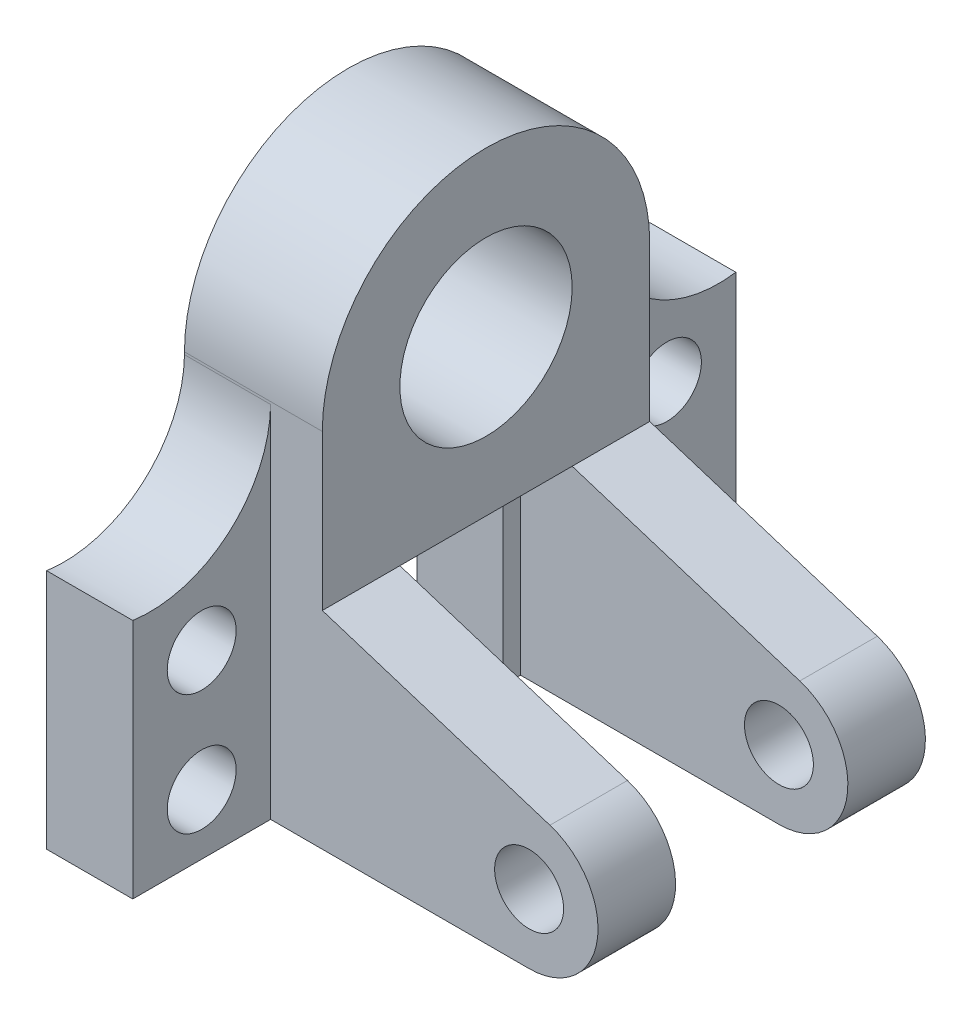
ISO-10303-21;
HEADER;
FILE_DESCRIPTION(('STEP AP214'),'2;1');
FILE_NAME('part.step','',(''),(''),'','','');
FILE_SCHEMA(('AUTOMOTIVE_DESIGN { 1 0 10303 214 1 1 1 1 }'));
ENDSEC;
DATA;
#1=APPLICATION_CONTEXT('core data for automotive mechanical design processes');
#2=APPLICATION_PROTOCOL_DEFINITION('international standard','automotive_design',2000,#1);
#3=PRODUCT_CONTEXT('',#1,'mechanical');
#4=PRODUCT('Part','Part','',(#3));
#5=PRODUCT_RELATED_PRODUCT_CATEGORY('part','',(#4));
#6=PRODUCT_DEFINITION_FORMATION('','',#4);
#7=PRODUCT_DEFINITION_CONTEXT('part definition',#1,'design');
#8=PRODUCT_DEFINITION('design','',#6,#7);
#9=PRODUCT_DEFINITION_SHAPE('','',#8);
#10=(LENGTH_UNIT() NAMED_UNIT(*) SI_UNIT(.MILLI.,.METRE.));
#11=(NAMED_UNIT(*) PLANE_ANGLE_UNIT() SI_UNIT($,.RADIAN.));
#12=(NAMED_UNIT(*) SI_UNIT($,.STERADIAN.) SOLID_ANGLE_UNIT());
#13=UNCERTAINTY_MEASURE_WITH_UNIT(LENGTH_MEASURE(1.E-05),#10,'distance_accuracy_value','');
#14=(GEOMETRIC_REPRESENTATION_CONTEXT(3) GLOBAL_UNCERTAINTY_ASSIGNED_CONTEXT((#13)) GLOBAL_UNIT_ASSIGNED_CONTEXT((#10,
#11,#12)) REPRESENTATION_CONTEXT('',''));
#15=CARTESIAN_POINT('',(0.,0.,0.));
#16=DIRECTION('',(0.,0.,1.));
#17=DIRECTION('',(1.,0.,0.));
#18=AXIS2_PLACEMENT_3D('',#15,#16,#17);
#19=CARTESIAN_POINT('',(16.,-36.,38.));
#20=DIRECTION('',(0.,1.,0.));
#21=DIRECTION('',(0.,0.,1.));
#22=AXIS2_PLACEMENT_3D('',#19,#20,#21);
#23=PLANE('',#22);
#24=DIRECTION('',(-1.,0.,0.));
#25=VECTOR('',#24,1.);
#26=CARTESIAN_POINT('',(4.,-36.,16.));
#27=LINE('',#26,#25);
#28=CARTESIAN_POINT('',(4.,-36.,16.));
#29=VERTEX_POINT('',#28);
#30=CARTESIAN_POINT('',(-16.,-36.,16.));
#31=VERTEX_POINT('',#30);
#32=EDGE_CURVE('E401',#29,#31,#27,.T.);
#33=ORIENTED_EDGE('',*,*,#32,.T.);
#34=DIRECTION('',(0.,0.,-1.));
#35=VECTOR('',#34,1.);
#36=CARTESIAN_POINT('',(-16.,-36.,38.));
#37=LINE('',#36,#35);
#38=CARTESIAN_POINT('',(-16.,-36.,-16.));
#39=VERTEX_POINT('',#38);
#40=EDGE_CURVE('E61',#31,#39,#37,.T.);
#41=ORIENTED_EDGE('',*,*,#40,.T.);
#42=DIRECTION('',(-1.,0.,0.));
#43=VECTOR('',#42,1.);
#44=CARTESIAN_POINT('',(4.,-36.,-16.));
#45=LINE('',#44,#43);
#46=CARTESIAN_POINT('',(4.,-36.,-16.));
#47=VERTEX_POINT('',#46);
#48=EDGE_CURVE('E57',#47,#39,#45,.T.);
#49=ORIENTED_EDGE('',*,*,#48,.F.);
#50=DIRECTION('',(0.,0.,1.));
#51=VECTOR('',#50,1.);
#52=CARTESIAN_POINT('',(4.,-36.,0.));
#53=LINE('',#52,#51);
#54=CARTESIAN_POINT('',(4.,-36.,-20.));
#55=VERTEX_POINT('',#54);
#56=EDGE_CURVE('E387',#55,#47,#53,.T.);
#57=ORIENTED_EDGE('',*,*,#56,.F.);
#58=DIRECTION('',(1.,0.,0.));
#59=VECTOR('',#58,1.);
#60=CARTESIAN_POINT('',(0.,-36.,-20.));
#61=LINE('',#60,#59);
#62=CARTESIAN_POINT('',(16.,-36.,-20.));
#63=VERTEX_POINT('',#62);
#64=EDGE_CURVE('E363',#55,#63,#61,.T.);
#65=ORIENTED_EDGE('',*,*,#64,.T.);
#66=DIRECTION('',(0.,0.,-1.));
#67=VECTOR('',#66,1.);
#68=CARTESIAN_POINT('',(16.,-36.,38.));
#69=LINE('',#68,#67);
#70=CARTESIAN_POINT('',(16.,-36.,20.));
#71=VERTEX_POINT('',#70);
#72=EDGE_CURVE('E250',#71,#63,#69,.T.);
#73=ORIENTED_EDGE('',*,*,#72,.F.);
#74=DIRECTION('',(1.,0.,0.));
#75=VECTOR('',#74,1.);
#76=CARTESIAN_POINT('',(0.,-36.,20.));
#77=LINE('',#76,#75);
#78=CARTESIAN_POINT('',(4.,-36.,20.));
#79=VERTEX_POINT('',#78);
#80=EDGE_CURVE('E208',#79,#71,#77,.T.);
#81=ORIENTED_EDGE('',*,*,#80,.F.);
#82=DIRECTION('',(0.,0.,-1.));
#83=VECTOR('',#82,1.);
#84=CARTESIAN_POINT('',(4.,-36.,0.));
#85=LINE('',#84,#83);
#86=EDGE_CURVE('E200',#79,#29,#85,.T.);
#87=ORIENTED_EDGE('',*,*,#86,.T.);
#88=EDGE_LOOP('',(#33,#41,#49,#57,#65,#73,#81,#87));
#89=FACE_BOUND('',#88,.T.);
#90=ADVANCED_FACE('F41',(#89),#23,.F.);
#91=CARTESIAN_POINT('',(0.,0.,20.));
#92=DIRECTION('',(0.,0.,1.));
#93=DIRECTION('',(1.,0.,0.));
#94=AXIS2_PLACEMENT_3D('',#91,#92,#93);
#95=PLANE('',#94);
#96=CARTESIAN_POINT('',(64.,-68.,20.));
#97=DIRECTION('',(0.,0.,1.));
#98=DIRECTION('',(1.,0.,0.));
#99=AXIS2_PLACEMENT_3D('',#96,#97,#98);
#100=CIRCLE('',#99,7.99999999999999);
#101=CARTESIAN_POINT('',(72.,-68.,20.));
#102=VERTEX_POINT('',#101);
#103=EDGE_CURVE('E210',#102,#102,#100,.T.);
#104=ORIENTED_EDGE('',*,*,#103,.T.);
#105=EDGE_LOOP('',(#104));
#106=FACE_BOUND('',#105,.T.);
#107=DIRECTION('',(0.,1.,0.));
#108=VECTOR('',#107,1.);
#109=CARTESIAN_POINT('',(4.,0.,20.));
#110=LINE('',#109,#108);
#111=CARTESIAN_POINT('',(4.,-84.,20.));
#112=VERTEX_POINT('',#111);
#113=EDGE_CURVE('E191',#112,#79,#110,.T.);
#114=ORIENTED_EDGE('',*,*,#113,.T.);
#115=ORIENTED_EDGE('',*,*,#80,.T.);
#116=DIRECTION('',(0.953254218877944,-0.302169479251962,0.));
#117=VECTOR('',#116,1.);
#118=CARTESIAN_POINT('',(-8.90869360580859,-28.1042605145002,20.));
#119=LINE('',#118,#117);
#120=CARTESIAN_POINT('',(68.8347116680314,-52.7479324979529,20.));
#121=VERTEX_POINT('',#120);
#122=EDGE_CURVE('E213',#71,#121,#119,.T.);
#123=ORIENTED_EDGE('',*,*,#122,.T.);
#124=CARTESIAN_POINT('',(64.,-68.,20.));
#125=DIRECTION('',(0.,0.,1.));
#126=DIRECTION('',(1.,0.,0.));
#127=AXIS2_PLACEMENT_3D('',#124,#125,#126);
#128=CIRCLE('',#127,16.);
#129=CARTESIAN_POINT('',(64.,-84.,20.));
#130=VERTEX_POINT('',#129);
#131=EDGE_CURVE('E202',#121,#130,#128,.F.);
#132=ORIENTED_EDGE('',*,*,#131,.T.);
#133=DIRECTION('',(1.,0.,0.));
#134=VECTOR('',#133,1.);
#135=CARTESIAN_POINT('',(0.,-84.,20.));
#136=LINE('',#135,#134);
#137=EDGE_CURVE('E187',#112,#130,#136,.T.);
#138=ORIENTED_EDGE('',*,*,#137,.F.);
#139=EDGE_LOOP('',(#114,#115,#123,#132,#138));
#140=FACE_BOUND('',#139,.T.);
#141=ADVANCED_FACE('F201',(#106,#140),#95,.F.);
#142=CARTESIAN_POINT('',(0.,0.,-20.));
#143=DIRECTION('',(0.,0.,-1.));
#144=DIRECTION('',(1.,0.,0.));
#145=AXIS2_PLACEMENT_3D('',#142,#143,#144);
#146=PLANE('',#145);
#147=CARTESIAN_POINT('',(64.,-68.,-20.));
#148=DIRECTION('',(0.,0.,1.));
#149=DIRECTION('',(1.,0.,0.));
#150=AXIS2_PLACEMENT_3D('',#147,#148,#149);
#151=CIRCLE('',#150,7.99999999999999);
#152=CARTESIAN_POINT('',(72.,-68.,-20.));
#153=VERTEX_POINT('',#152);
#154=EDGE_CURVE('E314',#153,#153,#151,.T.);
#155=ORIENTED_EDGE('',*,*,#154,.F.);
#156=EDGE_LOOP('',(#155));
#157=FACE_BOUND('',#156,.T.);
#158=DIRECTION('',(0.,1.,0.));
#159=VECTOR('',#158,1.);
#160=CARTESIAN_POINT('',(4.,0.,-20.));
#161=LINE('',#160,#159);
#162=CARTESIAN_POINT('',(4.,-84.,-20.));
#163=VERTEX_POINT('',#162);
#164=EDGE_CURVE('E378',#163,#55,#161,.T.);
#165=ORIENTED_EDGE('',*,*,#164,.F.);
#166=DIRECTION('',(1.,0.,0.));
#167=VECTOR('',#166,1.);
#168=CARTESIAN_POINT('',(0.,-84.,-20.));
#169=LINE('',#168,#167);
#170=CARTESIAN_POINT('',(64.,-84.,-20.));
#171=VERTEX_POINT('',#170);
#172=EDGE_CURVE('E357',#163,#171,#169,.T.);
#173=ORIENTED_EDGE('',*,*,#172,.T.);
#174=CARTESIAN_POINT('',(64.,-68.,-20.));
#175=DIRECTION('',(0.,0.,1.));
#176=DIRECTION('',(1.,0.,0.));
#177=AXIS2_PLACEMENT_3D('',#174,#175,#176);
#178=CIRCLE('',#177,16.);
#179=CARTESIAN_POINT('',(68.8347116680314,-52.7479324979529,-20.));
#180=VERTEX_POINT('',#179);
#181=EDGE_CURVE('E305',#180,#171,#178,.F.);
#182=ORIENTED_EDGE('',*,*,#181,.F.);
#183=DIRECTION('',(0.953254218877944,-0.302169479251962,0.));
#184=VECTOR('',#183,1.);
#185=CARTESIAN_POINT('',(-8.90869360580859,-28.1042605145002,-20.));
#186=LINE('',#185,#184);
#187=EDGE_CURVE('E361',#63,#180,#186,.T.);
#188=ORIENTED_EDGE('',*,*,#187,.F.);
#189=ORIENTED_EDGE('',*,*,#64,.F.);
#190=EDGE_LOOP('',(#165,#173,#182,#188,#189));
#191=FACE_BOUND('',#190,.T.);
#192=ADVANCED_FACE('F375',(#157,#191),#146,.F.);
#193=CARTESIAN_POINT('',(16.,0.,38.));
#194=DIRECTION('',(0.,0.,-1.));
#195=DIRECTION('',(0.,1.,0.));
#196=AXIS2_PLACEMENT_3D('',#193,#194,#195);
#197=PLANE('',#196);
#198=CARTESIAN_POINT('',(64.,-68.,38.));
#199=DIRECTION('',(0.,0.,1.));
#200=DIRECTION('',(1.,0.,0.));
#201=AXIS2_PLACEMENT_3D('',#198,#199,#200);
#202=CIRCLE('',#201,7.99999999999999);
#203=CARTESIAN_POINT('',(72.,-68.,38.));
#204=VERTEX_POINT('',#203);
#205=EDGE_CURVE('E223',#204,#204,#202,.T.);
#206=ORIENTED_EDGE('',*,*,#205,.F.);
#207=EDGE_LOOP('',(#206));
#208=FACE_BOUND('',#207,.T.);
#209=DIRECTION('',(-1.,0.,0.));
#210=VECTOR('',#209,1.);
#211=CARTESIAN_POINT('',(4.,-0.574800038644198,38.));
#212=LINE('',#211,#210);
#213=CARTESIAN_POINT('',(4.,-0.574800038644198,38.));
#214=VERTEX_POINT('',#213);
#215=CARTESIAN_POINT('',(-16.,-0.574800038644198,38.));
#216=VERTEX_POINT('',#215);
#217=EDGE_CURVE('E328',#214,#216,#212,.T.);
#218=ORIENTED_EDGE('',*,*,#217,.F.);
#219=DIRECTION('',(0.,1.,0.));
#220=VECTOR('',#219,1.);
#221=CARTESIAN_POINT('',(4.,0.,38.));
#222=LINE('',#221,#220);
#223=CARTESIAN_POINT('',(4.,-84.,38.));
#224=VERTEX_POINT('',#223);
#225=EDGE_CURVE('E327',#224,#214,#222,.T.);
#226=ORIENTED_EDGE('',*,*,#225,.F.);
#227=DIRECTION('',(1.,0.,0.));
#228=VECTOR('',#227,1.);
#229=CARTESIAN_POINT('',(0.,-84.,38.));
#230=LINE('',#229,#228);
#231=CARTESIAN_POINT('',(64.,-84.,38.));
#232=VERTEX_POINT('',#231);
#233=EDGE_CURVE('E224',#224,#232,#230,.T.);
#234=ORIENTED_EDGE('',*,*,#233,.T.);
#235=CARTESIAN_POINT('',(64.,-68.,38.));
#236=DIRECTION('',(0.,0.,1.));
#237=DIRECTION('',(1.,0.,0.));
#238=AXIS2_PLACEMENT_3D('',#235,#236,#237);
#239=CIRCLE('',#238,16.);
#240=CARTESIAN_POINT('',(68.8347116680314,-52.7479324979529,38.));
#241=VERTEX_POINT('',#240);
#242=EDGE_CURVE('E220',#241,#232,#239,.F.);
#243=ORIENTED_EDGE('',*,*,#242,.F.);
#244=DIRECTION('',(0.953254218877944,-0.302169479251962,0.));
#245=VECTOR('',#244,1.);
#246=CARTESIAN_POINT('',(-8.90869360580859,-28.1042605145002,38.));
#247=LINE('',#246,#245);
#248=CARTESIAN_POINT('',(16.,-36.,38.));
#249=VERTEX_POINT('',#248);
#250=EDGE_CURVE('E219',#249,#241,#247,.T.);
#251=ORIENTED_EDGE('',*,*,#250,.F.);
#252=DIRECTION('',(0.,-1.,0.));
#253=VECTOR('',#252,1.);
#254=CARTESIAN_POINT('',(16.,0.,38.));
#255=LINE('',#254,#253);
#256=CARTESIAN_POINT('',(16.,0.,38.));
#257=VERTEX_POINT('',#256);
#258=EDGE_CURVE('E243',#257,#249,#255,.T.);
#259=ORIENTED_EDGE('',*,*,#258,.F.);
#260=DIRECTION('',(-1.,0.,0.));
#261=VECTOR('',#260,1.);
#262=CARTESIAN_POINT('',(16.,0.,38.));
#263=LINE('',#262,#261);
#264=CARTESIAN_POINT('',(-16.,0.,38.));
#265=VERTEX_POINT('',#264);
#266=EDGE_CURVE('E11',#257,#265,#263,.T.);
#267=ORIENTED_EDGE('',*,*,#266,.T.);
#268=DIRECTION('',(0.,-1.,0.));
#269=VECTOR('',#268,1.);
#270=CARTESIAN_POINT('',(-16.,0.,38.));
#271=LINE('',#270,#269);
#272=EDGE_CURVE('E254',#265,#216,#271,.T.);
#273=ORIENTED_EDGE('',*,*,#272,.T.);
#274=EDGE_LOOP('',(#218,#226,#234,#243,#251,#259,#267,#273));
#275=FACE_BOUND('',#274,.T.);
#276=ADVANCED_FACE('F280',(#208,#275),#197,.F.);
#277=CARTESIAN_POINT('',(16.,0.,0.));
#278=DIRECTION('',(1.,0.,0.));
#279=DIRECTION('',(0.,0.,-1.));
#280=AXIS2_PLACEMENT_3D('',#277,#278,#279);
#281=PLANE('',#280);
#282=CARTESIAN_POINT('',(16.,0.,0.));
#283=DIRECTION('',(1.,0.,0.));
#284=DIRECTION('',(0.,0.,-1.));
#285=AXIS2_PLACEMENT_3D('',#282,#283,#284);
#286=CIRCLE('',#285,38.);
#287=CARTESIAN_POINT('',(16.,0.,-38.));
#288=VERTEX_POINT('',#287);
#289=EDGE_CURVE('E241',#288,#257,#286,.T.);
#290=ORIENTED_EDGE('',*,*,#289,.T.);
#291=ORIENTED_EDGE('',*,*,#258,.T.);
#292=EDGE_CURVE('E246',#249,#71,#69,.T.);
#293=ORIENTED_EDGE('',*,*,#292,.T.);
#294=ORIENTED_EDGE('',*,*,#72,.T.);
#295=DIRECTION('',(0.,0.,-1.));
#296=VECTOR('',#295,1.);
#297=CARTESIAN_POINT('',(16.,-36.,-20.));
#298=LINE('',#297,#296);
#299=CARTESIAN_POINT('',(16.,-36.,-38.));
#300=VERTEX_POINT('',#299);
#301=EDGE_CURVE('E290',#63,#300,#298,.T.);
#302=ORIENTED_EDGE('',*,*,#301,.T.);
#303=DIRECTION('',(0.,1.,0.));
#304=VECTOR('',#303,1.);
#305=CARTESIAN_POINT('',(16.,-36.,-38.));
#306=LINE('',#305,#304);
#307=EDGE_CURVE('E253',#300,#288,#306,.T.);
#308=ORIENTED_EDGE('',*,*,#307,.T.);
#309=EDGE_LOOP('',(#290,#291,#293,#294,#302,#308));
#310=FACE_BOUND('',#309,.T.);
#311=CARTESIAN_POINT('',(16.,0.,0.));
#312=DIRECTION('',(1.,0.,0.));
#313=DIRECTION('',(0.,0.,-1.));
#314=AXIS2_PLACEMENT_3D('',#311,#312,#313);
#315=CIRCLE('',#314,20.);
#316=CARTESIAN_POINT('',(16.,0.,-20.));
#317=VERTEX_POINT('',#316);
#318=EDGE_CURVE('E234',#317,#317,#315,.T.);
#319=ORIENTED_EDGE('',*,*,#318,.F.);
#320=EDGE_LOOP('',(#319));
#321=FACE_BOUND('',#320,.T.);
#322=ADVANCED_FACE('F285',(#310,#321),#281,.T.);
#323=CARTESIAN_POINT('',(-16.,0.,0.));
#324=DIRECTION('',(1.,0.,0.));
#325=DIRECTION('',(0.,0.,-1.));
#326=AXIS2_PLACEMENT_3D('',#323,#324,#325);
#327=PLANE('',#326);
#328=ORIENTED_EDGE('',*,*,#40,.F.);
#329=DIRECTION('',(0.,1.,0.));
#330=VECTOR('',#329,1.);
#331=CARTESIAN_POINT('',(-16.,0.,16.));
#332=LINE('',#331,#330);
#333=CARTESIAN_POINT('',(-16.,-84.,16.));
#334=VERTEX_POINT('',#333);
#335=EDGE_CURVE('E192',#334,#31,#332,.T.);
#336=ORIENTED_EDGE('',*,*,#335,.F.);
#337=DIRECTION('',(0.,0.,1.));
#338=VECTOR('',#337,1.);
#339=CARTESIAN_POINT('',(-16.,-84.,20.));
#340=LINE('',#339,#338);
#341=CARTESIAN_POINT('',(-16.,-84.,70.));
#342=VERTEX_POINT('',#341);
#343=EDGE_CURVE('E233',#334,#342,#340,.T.);
#344=ORIENTED_EDGE('',*,*,#343,.T.);
#345=DIRECTION('',(0.,1.,0.));
#346=VECTOR('',#345,1.);
#347=CARTESIAN_POINT('',(-16.,0.,70.));
#348=LINE('',#347,#346);
#349=CARTESIAN_POINT('',(-16.,-28.,70.));
#350=VERTEX_POINT('',#349);
#351=EDGE_CURVE('E349',#342,#350,#348,.T.);
#352=ORIENTED_EDGE('',*,*,#351,.T.);
#353=CARTESIAN_POINT('',(-16.,-0.287400019322068,65.9985249830932));
#354=DIRECTION('',(-1.,0.,0.));
#355=DIRECTION('',(0.,0.,1.));
#356=AXIS2_PLACEMENT_3D('',#353,#354,#355);
#357=CIRCLE('',#356,28.);
#358=EDGE_CURVE('E273',#216,#350,#357,.T.);
#359=ORIENTED_EDGE('',*,*,#358,.F.);
#360=ORIENTED_EDGE('',*,*,#272,.F.);
#361=CARTESIAN_POINT('',(-16.,0.,0.));
#362=DIRECTION('',(1.,0.,0.));
#363=DIRECTION('',(0.,0.,-1.));
#364=AXIS2_PLACEMENT_3D('',#361,#362,#363);
#365=CIRCLE('',#364,38.);
#366=CARTESIAN_POINT('',(-16.,0.,-38.));
#367=VERTEX_POINT('',#366);
#368=EDGE_CURVE('E236',#367,#265,#365,.T.);
#369=ORIENTED_EDGE('',*,*,#368,.F.);
#370=DIRECTION('',(0.,1.,0.));
#371=VECTOR('',#370,1.);
#372=CARTESIAN_POINT('',(-16.,-36.,-38.));
#373=LINE('',#372,#371);
#374=CARTESIAN_POINT('',(-16.,-0.574800038644198,-38.));
#375=VERTEX_POINT('',#374);
#376=EDGE_CURVE('E244',#375,#367,#373,.T.);
#377=ORIENTED_EDGE('',*,*,#376,.F.);
#378=CARTESIAN_POINT('',(-16.,-0.287400019322068,-65.9985249830932));
#379=DIRECTION('',(1.,0.,0.));
#380=DIRECTION('',(0.,0.,-1.));
#381=AXIS2_PLACEMENT_3D('',#378,#379,#380);
#382=CIRCLE('',#381,28.);
#383=CARTESIAN_POINT('',(-16.,-28.,-70.));
#384=VERTEX_POINT('',#383);
#385=EDGE_CURVE('E433',#375,#384,#382,.T.);
#386=ORIENTED_EDGE('',*,*,#385,.T.);
#387=DIRECTION('',(0.,1.,0.));
#388=VECTOR('',#387,1.);
#389=CARTESIAN_POINT('',(-16.,0.,-70.));
#390=LINE('',#389,#388);
#391=CARTESIAN_POINT('',(-16.,-84.,-70.));
#392=VERTEX_POINT('',#391);
#393=EDGE_CURVE('E412',#392,#384,#390,.T.);
#394=ORIENTED_EDGE('',*,*,#393,.F.);
#395=DIRECTION('',(0.,0.,-1.));
#396=VECTOR('',#395,1.);
#397=CARTESIAN_POINT('',(-16.,-84.,-20.));
#398=LINE('',#397,#396);
#399=CARTESIAN_POINT('',(-16.,-84.,-16.));
#400=VERTEX_POINT('',#399);
#401=EDGE_CURVE('E310',#400,#392,#398,.T.);
#402=ORIENTED_EDGE('',*,*,#401,.F.);
#403=DIRECTION('',(0.,1.,0.));
#404=VECTOR('',#403,1.);
#405=CARTESIAN_POINT('',(-16.,0.,-16.));
#406=LINE('',#405,#404);
#407=EDGE_CURVE('E400',#400,#39,#406,.T.);
#408=ORIENTED_EDGE('',*,*,#407,.T.);
#409=EDGE_LOOP('',(#328,#336,#344,#352,#359,#360,#369,#377,#386,#394,#402,#408));
#410=FACE_BOUND('',#409,.T.);
#411=CARTESIAN_POINT('',(-16.,0.,0.));
#412=DIRECTION('',(1.,0.,0.));
#413=DIRECTION('',(0.,0.,-1.));
#414=AXIS2_PLACEMENT_3D('',#411,#412,#413);
#415=CIRCLE('',#414,20.);
#416=CARTESIAN_POINT('',(-16.,0.,-20.));
#417=VERTEX_POINT('',#416);
#418=EDGE_CURVE('E229',#417,#417,#415,.T.);
#419=ORIENTED_EDGE('',*,*,#418,.T.);
#420=EDGE_LOOP('',(#419));
#421=FACE_BOUND('',#420,.T.);
#422=CARTESIAN_POINT('',(-16.,-70.,54.));
#423=DIRECTION('',(-1.,0.,0.));
#424=DIRECTION('',(0.,0.,1.));
#425=AXIS2_PLACEMENT_3D('',#422,#423,#424);
#426=CIRCLE('',#425,8.);
#427=CARTESIAN_POINT('',(-16.,-70.,62.));
#428=VERTEX_POINT('',#427);
#429=EDGE_CURVE('E343',#428,#428,#426,.T.);
#430=ORIENTED_EDGE('',*,*,#429,.F.);
#431=EDGE_LOOP('',(#430));
#432=FACE_BOUND('',#431,.T.);
#433=CARTESIAN_POINT('',(-16.,-42.,54.));
#434=DIRECTION('',(-1.,0.,0.));
#435=DIRECTION('',(0.,0.,1.));
#436=AXIS2_PLACEMENT_3D('',#433,#434,#435);
#437=CIRCLE('',#436,8.);
#438=CARTESIAN_POINT('',(-16.,-42.,62.));
#439=VERTEX_POINT('',#438);
#440=EDGE_CURVE('E342',#439,#439,#437,.T.);
#441=ORIENTED_EDGE('',*,*,#440,.F.);
#442=EDGE_LOOP('',(#441));
#443=FACE_BOUND('',#442,.T.);
#444=CARTESIAN_POINT('',(-16.,-70.,-54.));
#445=DIRECTION('',(1.,0.,0.));
#446=DIRECTION('',(0.,0.,-1.));
#447=AXIS2_PLACEMENT_3D('',#444,#445,#446);
#448=CIRCLE('',#447,8.);
#449=CARTESIAN_POINT('',(-16.,-70.,-62.));
#450=VERTEX_POINT('',#449);
#451=EDGE_CURVE('E407',#450,#450,#448,.T.);
#452=ORIENTED_EDGE('',*,*,#451,.T.);
#453=EDGE_LOOP('',(#452));
#454=FACE_BOUND('',#453,.T.);
#455=CARTESIAN_POINT('',(-16.,-42.,-54.));
#456=DIRECTION('',(1.,0.,0.));
#457=DIRECTION('',(0.,0.,-1.));
#458=AXIS2_PLACEMENT_3D('',#455,#456,#457);
#459=CIRCLE('',#458,8.);
#460=CARTESIAN_POINT('',(-16.,-42.,-62.));
#461=VERTEX_POINT('',#460);
#462=EDGE_CURVE('E429',#461,#461,#459,.T.);
#463=ORIENTED_EDGE('',*,*,#462,.T.);
#464=EDGE_LOOP('',(#463));
#465=FACE_BOUND('',#464,.T.);
#466=ADVANCED_FACE('F268',(#410,#421,#432,#443,#454,#465),#327,.F.);
#467=CARTESIAN_POINT('',(16.,0.,0.));
#468=DIRECTION('',(-1.,0.,0.));
#469=DIRECTION('',(0.,0.,1.));
#470=AXIS2_PLACEMENT_3D('',#467,#468,#469);
#471=CYLINDRICAL_SURFACE('',#470,38.);
#472=ORIENTED_EDGE('',*,*,#368,.T.);
#473=ORIENTED_EDGE('',*,*,#266,.F.);
#474=ORIENTED_EDGE('',*,*,#289,.F.);
#475=DIRECTION('',(-1.,0.,0.));
#476=VECTOR('',#475,1.);
#477=CARTESIAN_POINT('',(16.,0.,-38.));
#478=LINE('',#477,#476);
#479=EDGE_CURVE('E47',#288,#367,#478,.T.);
#480=ORIENTED_EDGE('',*,*,#479,.T.);
#481=EDGE_LOOP('',(#472,#473,#474,#480));
#482=FACE_BOUND('',#481,.T.);
#483=ADVANCED_FACE('F43',(#482),#471,.T.);
#484=CARTESIAN_POINT('',(16.,-36.,-38.));
#485=DIRECTION('',(0.,0.,1.));
#486=DIRECTION('',(0.,-1.,0.));
#487=AXIS2_PLACEMENT_3D('',#484,#485,#486);
#488=PLANE('',#487);
#489=DIRECTION('',(0.,1.,0.));
#490=VECTOR('',#489,1.);
#491=CARTESIAN_POINT('',(4.,0.,-38.));
#492=LINE('',#491,#490);
#493=CARTESIAN_POINT('',(4.,-84.,-38.));
#494=VERTEX_POINT('',#493);
#495=CARTESIAN_POINT('',(4.,-0.574800038644198,-38.));
#496=VERTEX_POINT('',#495);
#497=EDGE_CURVE('E422',#494,#496,#492,.T.);
#498=ORIENTED_EDGE('',*,*,#497,.T.);
#499=DIRECTION('',(-1.,0.,0.));
#500=VECTOR('',#499,1.);
#501=CARTESIAN_POINT('',(4.,-0.574800038644198,-38.));
#502=LINE('',#501,#500);
#503=EDGE_CURVE('E344',#496,#375,#502,.T.);
#504=ORIENTED_EDGE('',*,*,#503,.T.);
#505=ORIENTED_EDGE('',*,*,#376,.T.);
#506=ORIENTED_EDGE('',*,*,#479,.F.);
#507=ORIENTED_EDGE('',*,*,#307,.F.);
#508=DIRECTION('',(0.953254218877944,-0.302169479251962,0.));
#509=VECTOR('',#508,1.);
#510=CARTESIAN_POINT('',(-8.90869360580859,-28.1042605145002,-38.));
#511=LINE('',#510,#509);
#512=CARTESIAN_POINT('',(68.8347116680314,-52.7479324979529,-38.));
#513=VERTEX_POINT('',#512);
#514=EDGE_CURVE('E291',#300,#513,#511,.T.);
#515=ORIENTED_EDGE('',*,*,#514,.T.);
#516=CARTESIAN_POINT('',(64.,-68.,-38.));
#517=DIRECTION('',(0.,0.,1.));
#518=DIRECTION('',(1.,0.,0.));
#519=AXIS2_PLACEMENT_3D('',#516,#517,#518);
#520=CIRCLE('',#519,16.);
#521=CARTESIAN_POINT('',(64.,-84.,-38.));
#522=VERTEX_POINT('',#521);
#523=EDGE_CURVE('E296',#513,#522,#520,.F.);
#524=ORIENTED_EDGE('',*,*,#523,.T.);
#525=DIRECTION('',(1.,0.,0.));
#526=VECTOR('',#525,1.);
#527=CARTESIAN_POINT('',(0.,-84.,-38.));
#528=LINE('',#527,#526);
#529=EDGE_CURVE('E298',#494,#522,#528,.T.);
#530=ORIENTED_EDGE('',*,*,#529,.F.);
#531=EDGE_LOOP('',(#498,#504,#505,#506,#507,#515,#524,#530));
#532=FACE_BOUND('',#531,.T.);
#533=CARTESIAN_POINT('',(64.,-68.,-38.));
#534=DIRECTION('',(0.,0.,1.));
#535=DIRECTION('',(1.,0.,0.));
#536=AXIS2_PLACEMENT_3D('',#533,#534,#535);
#537=CIRCLE('',#536,7.99999999999999);
#538=CARTESIAN_POINT('',(72.,-68.,-38.));
#539=VERTEX_POINT('',#538);
#540=EDGE_CURVE('E297',#539,#539,#537,.T.);
#541=ORIENTED_EDGE('',*,*,#540,.T.);
#542=EDGE_LOOP('',(#541));
#543=FACE_BOUND('',#542,.T.);
#544=ADVANCED_FACE('F289',(#532,#543),#488,.F.);
#545=CARTESIAN_POINT('',(16.,0.,0.));
#546=DIRECTION('',(-1.,0.,0.));
#547=DIRECTION('',(0.,0.,1.));
#548=AXIS2_PLACEMENT_3D('',#545,#546,#547);
#549=CYLINDRICAL_SURFACE('',#548,20.);
#550=ORIENTED_EDGE('',*,*,#318,.T.);
#551=EDGE_LOOP('',(#550));
#552=FACE_BOUND('',#551,.T.);
#553=ORIENTED_EDGE('',*,*,#418,.F.);
#554=EDGE_LOOP('',(#553));
#555=FACE_BOUND('',#554,.T.);
#556=ADVANCED_FACE('F498',(#552,#555),#549,.F.);
#557=CARTESIAN_POINT('',(64.,-68.,20.));
#558=DIRECTION('',(0.,0.,1.));
#559=DIRECTION('',(1.,0.,0.));
#560=AXIS2_PLACEMENT_3D('',#557,#558,#559);
#561=CYLINDRICAL_SURFACE('',#560,16.);
#562=ORIENTED_EDGE('',*,*,#242,.T.);
#563=DIRECTION('',(0.,0.,1.));
#564=VECTOR('',#563,1.);
#565=CARTESIAN_POINT('',(64.,-84.,20.));
#566=LINE('',#565,#564);
#567=EDGE_CURVE('E227',#130,#232,#566,.T.);
#568=ORIENTED_EDGE('',*,*,#567,.F.);
#569=ORIENTED_EDGE('',*,*,#131,.F.);
#570=DIRECTION('',(0.,0.,1.));
#571=VECTOR('',#570,1.);
#572=CARTESIAN_POINT('',(68.8347116680314,-52.7479324979529,20.));
#573=LINE('',#572,#571);
#574=EDGE_CURVE('E211',#121,#241,#573,.T.);
#575=ORIENTED_EDGE('',*,*,#574,.T.);
#576=EDGE_LOOP('',(#562,#568,#569,#575));
#577=FACE_BOUND('',#576,.T.);
#578=ADVANCED_FACE('F319',(#577),#561,.T.);
#579=CARTESIAN_POINT('',(0.,-84.,20.));
#580=DIRECTION('',(0.,-1.,0.));
#581=DIRECTION('',(0.,0.,-1.));
#582=AXIS2_PLACEMENT_3D('',#579,#580,#581);
#583=PLANE('',#582);
#584=ORIENTED_EDGE('',*,*,#233,.F.);
#585=DIRECTION('',(0.,0.,1.));
#586=VECTOR('',#585,1.);
#587=CARTESIAN_POINT('',(4.,-84.,0.));
#588=LINE('',#587,#586);
#589=CARTESIAN_POINT('',(4.,-84.,70.));
#590=VERTEX_POINT('',#589);
#591=EDGE_CURVE('E324',#224,#590,#588,.T.);
#592=ORIENTED_EDGE('',*,*,#591,.T.);
#593=DIRECTION('',(-1.,0.,0.));
#594=VECTOR('',#593,1.);
#595=CARTESIAN_POINT('',(4.,-84.,70.));
#596=LINE('',#595,#594);
#597=EDGE_CURVE('E353',#590,#342,#596,.T.);
#598=ORIENTED_EDGE('',*,*,#597,.T.);
#599=ORIENTED_EDGE('',*,*,#343,.F.);
#600=DIRECTION('',(-1.,0.,0.));
#601=VECTOR('',#600,1.);
#602=CARTESIAN_POINT('',(4.,-84.,16.));
#603=LINE('',#602,#601);
#604=CARTESIAN_POINT('',(4.,-84.,16.));
#605=VERTEX_POINT('',#604);
#606=EDGE_CURVE('E193',#605,#334,#603,.T.);
#607=ORIENTED_EDGE('',*,*,#606,.F.);
#608=DIRECTION('',(0.,0.,-1.));
#609=VECTOR('',#608,1.);
#610=CARTESIAN_POINT('',(4.,-84.,0.));
#611=LINE('',#610,#609);
#612=EDGE_CURVE('E181',#112,#605,#611,.T.);
#613=ORIENTED_EDGE('',*,*,#612,.F.);
#614=ORIENTED_EDGE('',*,*,#137,.T.);
#615=ORIENTED_EDGE('',*,*,#567,.T.);
#616=EDGE_LOOP('',(#584,#592,#598,#599,#607,#613,#614,#615));
#617=FACE_BOUND('',#616,.T.);
#618=ADVANCED_FACE('F183',(#617),#583,.T.);
#619=CARTESIAN_POINT('',(-8.90869360580859,-28.1042605145002,20.));
#620=DIRECTION('',(-0.302169479251962,-0.953254218877943,0.));
#621=DIRECTION('',(0.953254218877943,-0.302169479251962,0.));
#622=AXIS2_PLACEMENT_3D('',#619,#620,#621);
#623=PLANE('',#622);
#624=ORIENTED_EDGE('',*,*,#250,.T.);
#625=ORIENTED_EDGE('',*,*,#574,.F.);
#626=ORIENTED_EDGE('',*,*,#122,.F.);
#627=ORIENTED_EDGE('',*,*,#292,.F.);
#628=EDGE_LOOP('',(#624,#625,#626,#627));
#629=FACE_BOUND('',#628,.T.);
#630=ADVANCED_FACE('F318',(#629),#623,.F.);
#631=CARTESIAN_POINT('',(64.,-68.,20.));
#632=DIRECTION('',(0.,0.,1.));
#633=DIRECTION('',(1.,0.,0.));
#634=AXIS2_PLACEMENT_3D('',#631,#632,#633);
#635=CYLINDRICAL_SURFACE('',#634,7.99999999999999);
#636=ORIENTED_EDGE('',*,*,#103,.F.);
#637=EDGE_LOOP('',(#636));
#638=FACE_BOUND('',#637,.T.);
#639=ORIENTED_EDGE('',*,*,#205,.T.);
#640=EDGE_LOOP('',(#639));
#641=FACE_BOUND('',#640,.T.);
#642=ADVANCED_FACE('F468',(#638,#641),#635,.F.);
#643=CARTESIAN_POINT('',(64.,-68.,-20.));
#644=DIRECTION('',(0.,0.,-1.));
#645=DIRECTION('',(-1.,0.,0.));
#646=AXIS2_PLACEMENT_3D('',#643,#644,#645);
#647=CYLINDRICAL_SURFACE('',#646,16.);
#648=ORIENTED_EDGE('',*,*,#523,.F.);
#649=DIRECTION('',(0.,0.,-1.));
#650=VECTOR('',#649,1.);
#651=CARTESIAN_POINT('',(68.8347116680314,-52.7479324979529,-20.));
#652=LINE('',#651,#650);
#653=EDGE_CURVE('E222',#180,#513,#652,.T.);
#654=ORIENTED_EDGE('',*,*,#653,.F.);
#655=ORIENTED_EDGE('',*,*,#181,.T.);
#656=DIRECTION('',(0.,0.,-1.));
#657=VECTOR('',#656,1.);
#658=CARTESIAN_POINT('',(64.,-84.,-20.));
#659=LINE('',#658,#657);
#660=EDGE_CURVE('E313',#171,#522,#659,.T.);
#661=ORIENTED_EDGE('',*,*,#660,.T.);
#662=EDGE_LOOP('',(#648,#654,#655,#661));
#663=FACE_BOUND('',#662,.T.);
#664=ADVANCED_FACE('F463',(#663),#647,.T.);
#665=CARTESIAN_POINT('',(-8.90869360580859,-28.1042605145002,-20.));
#666=DIRECTION('',(0.302169479251962,0.953254218877943,0.));
#667=DIRECTION('',(-0.953254218877943,0.302169479251962,0.));
#668=AXIS2_PLACEMENT_3D('',#665,#666,#667);
#669=PLANE('',#668);
#670=ORIENTED_EDGE('',*,*,#514,.F.);
#671=ORIENTED_EDGE('',*,*,#301,.F.);
#672=ORIENTED_EDGE('',*,*,#187,.T.);
#673=ORIENTED_EDGE('',*,*,#653,.T.);
#674=EDGE_LOOP('',(#670,#671,#672,#673));
#675=FACE_BOUND('',#674,.T.);
#676=ADVANCED_FACE('F465',(#675),#669,.T.);
#677=CARTESIAN_POINT('',(0.,-84.,-20.));
#678=DIRECTION('',(0.,1.,0.));
#679=DIRECTION('',(0.,0.,1.));
#680=AXIS2_PLACEMENT_3D('',#677,#678,#679);
#681=PLANE('',#680);
#682=ORIENTED_EDGE('',*,*,#401,.T.);
#683=DIRECTION('',(-1.,0.,0.));
#684=VECTOR('',#683,1.);
#685=CARTESIAN_POINT('',(4.,-84.,-70.));
#686=LINE('',#685,#684);
#687=CARTESIAN_POINT('',(4.,-84.,-70.));
#688=VERTEX_POINT('',#687);
#689=EDGE_CURVE('E438',#688,#392,#686,.T.);
#690=ORIENTED_EDGE('',*,*,#689,.F.);
#691=DIRECTION('',(0.,0.,-1.));
#692=VECTOR('',#691,1.);
#693=CARTESIAN_POINT('',(4.,-84.,0.));
#694=LINE('',#693,#692);
#695=EDGE_CURVE('E425',#494,#688,#694,.T.);
#696=ORIENTED_EDGE('',*,*,#695,.F.);
#697=ORIENTED_EDGE('',*,*,#529,.T.);
#698=ORIENTED_EDGE('',*,*,#660,.F.);
#699=ORIENTED_EDGE('',*,*,#172,.F.);
#700=DIRECTION('',(0.,0.,1.));
#701=VECTOR('',#700,1.);
#702=CARTESIAN_POINT('',(4.,-84.,0.));
#703=LINE('',#702,#701);
#704=CARTESIAN_POINT('',(4.,-84.,-16.));
#705=VERTEX_POINT('',#704);
#706=EDGE_CURVE('E395',#163,#705,#703,.T.);
#707=ORIENTED_EDGE('',*,*,#706,.T.);
#708=DIRECTION('',(-1.,0.,0.));
#709=VECTOR('',#708,1.);
#710=CARTESIAN_POINT('',(4.,-84.,-16.));
#711=LINE('',#710,#709);
#712=EDGE_CURVE('E384',#705,#400,#711,.T.);
#713=ORIENTED_EDGE('',*,*,#712,.T.);
#714=EDGE_LOOP('',(#682,#690,#696,#697,#698,#699,#707,#713));
#715=FACE_BOUND('',#714,.T.);
#716=ADVANCED_FACE('F388',(#715),#681,.F.);
#717=CARTESIAN_POINT('',(64.,-68.,-20.));
#718=DIRECTION('',(0.,0.,-1.));
#719=DIRECTION('',(-1.,0.,0.));
#720=AXIS2_PLACEMENT_3D('',#717,#718,#719);
#721=CYLINDRICAL_SURFACE('',#720,7.99999999999999);
#722=ORIENTED_EDGE('',*,*,#154,.T.);
#723=EDGE_LOOP('',(#722));
#724=FACE_BOUND('',#723,.T.);
#725=ORIENTED_EDGE('',*,*,#540,.F.);
#726=EDGE_LOOP('',(#725));
#727=FACE_BOUND('',#726,.T.);
#728=ADVANCED_FACE('F369',(#724,#727),#721,.F.);
#729=CARTESIAN_POINT('',(4.,-0.287400019322068,65.9985249830932));
#730=DIRECTION('',(-1.,0.,0.));
#731=DIRECTION('',(0.,0.,1.));
#732=AXIS2_PLACEMENT_3D('',#729,#730,#731);
#733=CYLINDRICAL_SURFACE('',#732,28.);
#734=ORIENTED_EDGE('',*,*,#358,.T.);
#735=DIRECTION('',(-1.,0.,0.));
#736=VECTOR('',#735,1.);
#737=CARTESIAN_POINT('',(4.,-28.,70.));
#738=LINE('',#737,#736);
#739=CARTESIAN_POINT('',(4.,-28.,70.));
#740=VERTEX_POINT('',#739);
#741=EDGE_CURVE('E355',#740,#350,#738,.T.);
#742=ORIENTED_EDGE('',*,*,#741,.F.);
#743=CARTESIAN_POINT('',(4.,-0.287400019322068,65.9985249830932));
#744=DIRECTION('',(-1.,0.,0.));
#745=DIRECTION('',(0.,0.,1.));
#746=AXIS2_PLACEMENT_3D('',#743,#744,#745);
#747=CIRCLE('',#746,28.);
#748=EDGE_CURVE('E335',#214,#740,#747,.T.);
#749=ORIENTED_EDGE('',*,*,#748,.F.);
#750=ORIENTED_EDGE('',*,*,#217,.T.);
#751=EDGE_LOOP('',(#734,#742,#749,#750));
#752=FACE_BOUND('',#751,.T.);
#753=ADVANCED_FACE('F448',(#752),#733,.F.);
#754=CARTESIAN_POINT('',(4.,0.,70.));
#755=DIRECTION('',(0.,0.,1.));
#756=DIRECTION('',(1.,0.,0.));
#757=AXIS2_PLACEMENT_3D('',#754,#755,#756);
#758=PLANE('',#757);
#759=ORIENTED_EDGE('',*,*,#351,.F.);
#760=ORIENTED_EDGE('',*,*,#597,.F.);
#761=DIRECTION('',(0.,1.,0.));
#762=VECTOR('',#761,1.);
#763=CARTESIAN_POINT('',(4.,0.,70.));
#764=LINE('',#763,#762);
#765=EDGE_CURVE('E336',#590,#740,#764,.T.);
#766=ORIENTED_EDGE('',*,*,#765,.T.);
#767=ORIENTED_EDGE('',*,*,#741,.T.);
#768=EDGE_LOOP('',(#759,#760,#766,#767));
#769=FACE_BOUND('',#768,.T.);
#770=ADVANCED_FACE('F455',(#769),#758,.T.);
#771=CARTESIAN_POINT('',(4.,-42.,54.));
#772=DIRECTION('',(-1.,0.,0.));
#773=DIRECTION('',(0.,0.,1.));
#774=AXIS2_PLACEMENT_3D('',#771,#772,#773);
#775=CYLINDRICAL_SURFACE('',#774,8.);
#776=CARTESIAN_POINT('',(4.,-42.,54.));
#777=DIRECTION('',(-1.,0.,0.));
#778=DIRECTION('',(0.,0.,1.));
#779=AXIS2_PLACEMENT_3D('',#776,#777,#778);
#780=CIRCLE('',#779,8.);
#781=CARTESIAN_POINT('',(4.,-42.,62.));
#782=VERTEX_POINT('',#781);
#783=EDGE_CURVE('E443',#782,#782,#780,.T.);
#784=ORIENTED_EDGE('',*,*,#783,.F.);
#785=EDGE_LOOP('',(#784));
#786=FACE_BOUND('',#785,.T.);
#787=ORIENTED_EDGE('',*,*,#440,.T.);
#788=EDGE_LOOP('',(#787));
#789=FACE_BOUND('',#788,.T.);
#790=ADVANCED_FACE('F630',(#786,#789),#775,.F.);
#791=CARTESIAN_POINT('',(4.,-70.,54.));
#792=DIRECTION('',(-1.,0.,0.));
#793=DIRECTION('',(0.,0.,1.));
#794=AXIS2_PLACEMENT_3D('',#791,#792,#793);
#795=CYLINDRICAL_SURFACE('',#794,8.);
#796=CARTESIAN_POINT('',(4.,-70.,54.));
#797=DIRECTION('',(-1.,0.,0.));
#798=DIRECTION('',(0.,0.,1.));
#799=AXIS2_PLACEMENT_3D('',#796,#797,#798);
#800=CIRCLE('',#799,8.);
#801=CARTESIAN_POINT('',(4.,-70.,62.));
#802=VERTEX_POINT('',#801);
#803=EDGE_CURVE('E351',#802,#802,#800,.T.);
#804=ORIENTED_EDGE('',*,*,#803,.F.);
#805=EDGE_LOOP('',(#804));
#806=FACE_BOUND('',#805,.T.);
#807=ORIENTED_EDGE('',*,*,#429,.T.);
#808=EDGE_LOOP('',(#807));
#809=FACE_BOUND('',#808,.T.);
#810=ADVANCED_FACE('F620',(#806,#809),#795,.F.);
#811=CARTESIAN_POINT('',(4.,0.,0.));
#812=DIRECTION('',(-1.,0.,0.));
#813=DIRECTION('',(0.,0.,1.));
#814=AXIS2_PLACEMENT_3D('',#811,#812,#813);
#815=PLANE('',#814);
#816=ORIENTED_EDGE('',*,*,#803,.T.);
#817=EDGE_LOOP('',(#816));
#818=FACE_BOUND('',#817,.T.);
#819=ORIENTED_EDGE('',*,*,#783,.T.);
#820=EDGE_LOOP('',(#819));
#821=FACE_BOUND('',#820,.T.);
#822=ORIENTED_EDGE('',*,*,#748,.T.);
#823=ORIENTED_EDGE('',*,*,#765,.F.);
#824=ORIENTED_EDGE('',*,*,#591,.F.);
#825=ORIENTED_EDGE('',*,*,#225,.T.);
#826=EDGE_LOOP('',(#822,#823,#824,#825));
#827=FACE_BOUND('',#826,.T.);
#828=ADVANCED_FACE('F331',(#818,#821,#827),#815,.F.);
#829=CARTESIAN_POINT('',(4.,-0.287400019322068,-65.9985249830932));
#830=DIRECTION('',(-1.,0.,0.));
#831=DIRECTION('',(0.,0.,1.));
#832=AXIS2_PLACEMENT_3D('',#829,#830,#831);
#833=CYLINDRICAL_SURFACE('',#832,28.);
#834=ORIENTED_EDGE('',*,*,#385,.F.);
#835=ORIENTED_EDGE('',*,*,#503,.F.);
#836=CARTESIAN_POINT('',(4.,-0.287400019322068,-65.9985249830932));
#837=DIRECTION('',(1.,0.,0.));
#838=DIRECTION('',(0.,0.,-1.));
#839=AXIS2_PLACEMENT_3D('',#836,#837,#838);
#840=CIRCLE('',#839,28.);
#841=CARTESIAN_POINT('',(4.,-28.,-70.));
#842=VERTEX_POINT('',#841);
#843=EDGE_CURVE('E417',#496,#842,#840,.T.);
#844=ORIENTED_EDGE('',*,*,#843,.T.);
#845=DIRECTION('',(-1.,0.,0.));
#846=VECTOR('',#845,1.);
#847=CARTESIAN_POINT('',(4.,-28.,-70.));
#848=LINE('',#847,#846);
#849=EDGE_CURVE('E430',#842,#384,#848,.T.);
#850=ORIENTED_EDGE('',*,*,#849,.T.);
#851=EDGE_LOOP('',(#834,#835,#844,#850));
#852=FACE_BOUND('',#851,.T.);
#853=ADVANCED_FACE('F597',(#852),#833,.F.);
#854=CARTESIAN_POINT('',(4.,-42.,-54.));
#855=DIRECTION('',(-1.,0.,0.));
#856=DIRECTION('',(0.,0.,1.));
#857=AXIS2_PLACEMENT_3D('',#854,#855,#856);
#858=CYLINDRICAL_SURFACE('',#857,8.);
#859=CARTESIAN_POINT('',(4.,-42.,-54.));
#860=DIRECTION('',(1.,0.,0.));
#861=DIRECTION('',(0.,0.,-1.));
#862=AXIS2_PLACEMENT_3D('',#859,#860,#861);
#863=CIRCLE('',#862,8.);
#864=CARTESIAN_POINT('',(4.,-42.,-62.));
#865=VERTEX_POINT('',#864);
#866=EDGE_CURVE('E411',#865,#865,#863,.T.);
#867=ORIENTED_EDGE('',*,*,#866,.T.);
#868=EDGE_LOOP('',(#867));
#869=FACE_BOUND('',#868,.T.);
#870=ORIENTED_EDGE('',*,*,#462,.F.);
#871=EDGE_LOOP('',(#870));
#872=FACE_BOUND('',#871,.T.);
#873=ADVANCED_FACE('F587',(#869,#872),#858,.F.);
#874=CARTESIAN_POINT('',(4.,-70.,-54.));
#875=DIRECTION('',(-1.,0.,0.));
#876=DIRECTION('',(0.,0.,1.));
#877=AXIS2_PLACEMENT_3D('',#874,#875,#876);
#878=CYLINDRICAL_SURFACE('',#877,8.);
#879=CARTESIAN_POINT('',(4.,-70.,-54.));
#880=DIRECTION('',(1.,0.,0.));
#881=DIRECTION('',(0.,0.,-1.));
#882=AXIS2_PLACEMENT_3D('',#879,#880,#881);
#883=CIRCLE('',#882,8.);
#884=CARTESIAN_POINT('',(4.,-70.,-62.));
#885=VERTEX_POINT('',#884);
#886=EDGE_CURVE('E409',#885,#885,#883,.T.);
#887=ORIENTED_EDGE('',*,*,#886,.T.);
#888=EDGE_LOOP('',(#887));
#889=FACE_BOUND('',#888,.T.);
#890=ORIENTED_EDGE('',*,*,#451,.F.);
#891=EDGE_LOOP('',(#890));
#892=FACE_BOUND('',#891,.T.);
#893=ADVANCED_FACE('F583',(#889,#892),#878,.F.);
#894=CARTESIAN_POINT('',(4.,0.,-70.));
#895=DIRECTION('',(0.,0.,1.));
#896=DIRECTION('',(1.,0.,0.));
#897=AXIS2_PLACEMENT_3D('',#894,#895,#896);
#898=PLANE('',#897);
#899=ORIENTED_EDGE('',*,*,#393,.T.);
#900=ORIENTED_EDGE('',*,*,#849,.F.);
#901=DIRECTION('',(0.,1.,0.));
#902=VECTOR('',#901,1.);
#903=CARTESIAN_POINT('',(4.,0.,-70.));
#904=LINE('',#903,#902);
#905=EDGE_CURVE('E419',#688,#842,#904,.T.);
#906=ORIENTED_EDGE('',*,*,#905,.F.);
#907=ORIENTED_EDGE('',*,*,#689,.T.);
#908=EDGE_LOOP('',(#899,#900,#906,#907));
#909=FACE_BOUND('',#908,.T.);
#910=ADVANCED_FACE('F575',(#909),#898,.F.);
#911=CARTESIAN_POINT('',(4.,0.,0.));
#912=DIRECTION('',(-1.,0.,0.));
#913=DIRECTION('',(0.,0.,-1.));
#914=AXIS2_PLACEMENT_3D('',#911,#912,#913);
#915=PLANE('',#914);
#916=ORIENTED_EDGE('',*,*,#886,.F.);
#917=EDGE_LOOP('',(#916));
#918=FACE_BOUND('',#917,.T.);
#919=ORIENTED_EDGE('',*,*,#866,.F.);
#920=EDGE_LOOP('',(#919));
#921=FACE_BOUND('',#920,.T.);
#922=ORIENTED_EDGE('',*,*,#843,.F.);
#923=ORIENTED_EDGE('',*,*,#497,.F.);
#924=ORIENTED_EDGE('',*,*,#695,.T.);
#925=ORIENTED_EDGE('',*,*,#905,.T.);
#926=EDGE_LOOP('',(#922,#923,#924,#925));
#927=FACE_BOUND('',#926,.T.);
#928=ADVANCED_FACE('F551',(#918,#921,#927),#915,.F.);
#929=CARTESIAN_POINT('',(4.,0.,-16.));
#930=DIRECTION('',(0.,0.,1.));
#931=DIRECTION('',(1.,0.,0.));
#932=AXIS2_PLACEMENT_3D('',#929,#930,#931);
#933=PLANE('',#932);
#934=ORIENTED_EDGE('',*,*,#407,.F.);
#935=ORIENTED_EDGE('',*,*,#712,.F.);
#936=DIRECTION('',(0.,1.,0.));
#937=VECTOR('',#936,1.);
#938=CARTESIAN_POINT('',(4.,0.,-16.));
#939=LINE('',#938,#937);
#940=EDGE_CURVE('E398',#705,#47,#939,.T.);
#941=ORIENTED_EDGE('',*,*,#940,.T.);
#942=ORIENTED_EDGE('',*,*,#48,.T.);
#943=EDGE_LOOP('',(#934,#935,#941,#942));
#944=FACE_BOUND('',#943,.T.);
#945=ADVANCED_FACE('F546',(#944),#933,.T.);
#946=CARTESIAN_POINT('',(4.,0.,0.));
#947=DIRECTION('',(-1.,0.,0.));
#948=DIRECTION('',(0.,0.,1.));
#949=AXIS2_PLACEMENT_3D('',#946,#947,#948);
#950=PLANE('',#949);
#951=ORIENTED_EDGE('',*,*,#706,.F.);
#952=ORIENTED_EDGE('',*,*,#164,.T.);
#953=ORIENTED_EDGE('',*,*,#56,.T.);
#954=ORIENTED_EDGE('',*,*,#940,.F.);
#955=EDGE_LOOP('',(#951,#952,#953,#954));
#956=FACE_BOUND('',#955,.T.);
#957=ADVANCED_FACE('F393',(#956),#950,.F.);
#958=CARTESIAN_POINT('',(4.,0.,16.));
#959=DIRECTION('',(0.,0.,1.));
#960=DIRECTION('',(1.,0.,0.));
#961=AXIS2_PLACEMENT_3D('',#958,#959,#960);
#962=PLANE('',#961);
#963=ORIENTED_EDGE('',*,*,#335,.T.);
#964=ORIENTED_EDGE('',*,*,#32,.F.);
#965=DIRECTION('',(0.,1.,0.));
#966=VECTOR('',#965,1.);
#967=CARTESIAN_POINT('',(4.,0.,16.));
#968=LINE('',#967,#966);
#969=EDGE_CURVE('E456',#605,#29,#968,.T.);
#970=ORIENTED_EDGE('',*,*,#969,.F.);
#971=ORIENTED_EDGE('',*,*,#606,.T.);
#972=EDGE_LOOP('',(#963,#964,#970,#971));
#973=FACE_BOUND('',#972,.T.);
#974=ADVANCED_FACE('F460',(#973),#962,.F.);
#975=CARTESIAN_POINT('',(4.,0.,0.));
#976=DIRECTION('',(-1.,0.,0.));
#977=DIRECTION('',(0.,0.,-1.));
#978=AXIS2_PLACEMENT_3D('',#975,#976,#977);
#979=PLANE('',#978);
#980=ORIENTED_EDGE('',*,*,#612,.T.);
#981=ORIENTED_EDGE('',*,*,#969,.T.);
#982=ORIENTED_EDGE('',*,*,#86,.F.);
#983=ORIENTED_EDGE('',*,*,#113,.F.);
#984=EDGE_LOOP('',(#980,#981,#982,#983));
#985=FACE_BOUND('',#984,.T.);
#986=ADVANCED_FACE('F197',(#985),#979,.F.);
#987=CLOSED_SHELL('',(#90,#141,#192,#276,#322,#466,#483,#544,#556,#578,#618,#630,#642,#664,#676,
#716,#728,#753,#770,#790,#810,#828,#853,#873,#893,#910,#928,#945,#957,#974,#986));
#988=MANIFOLD_SOLID_BREP('B2',#987);
#989=ADVANCED_BREP_SHAPE_REPRESENTATION('',(#18,#988),#14);
#990=SHAPE_DEFINITION_REPRESENTATION(#9,#989);
ENDSEC;
END-ISO-10303-21;
